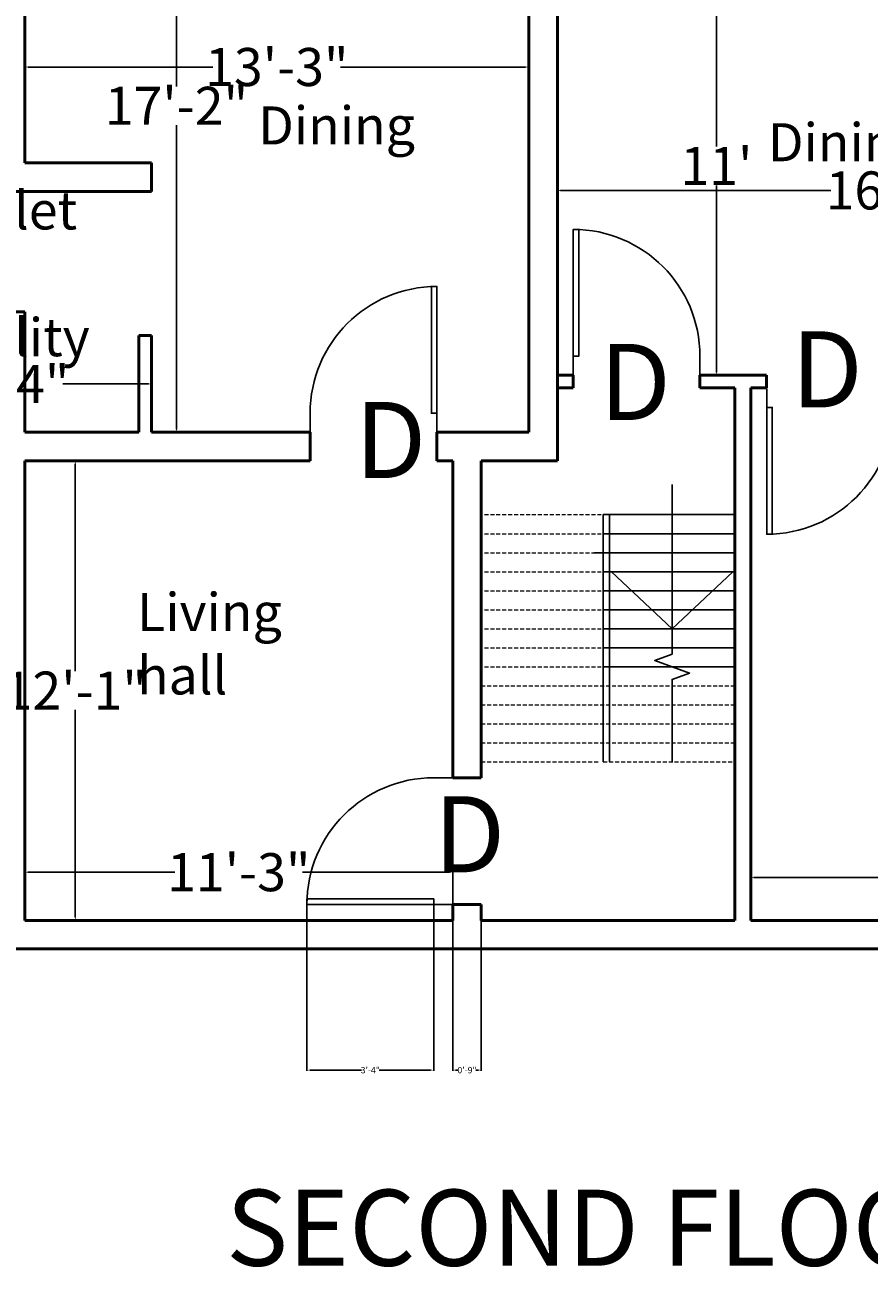
# Model space of a CAD drawing. Units: inches. Extents: x 409 to 7572, y 7 to 725.
# Tile 15 of 38: x 2984 to 3250, y 56 to 448. Entities that reach past the tile are written whole.
import ezdxf

# ---------------------------------------------------------------- set-up
doc = ezdxf.new("R2010")
doc.units = ezdxf.units.IN
doc.header["$MEASUREMENT"] = 0
doc.linetypes.add('HIDDEN', pattern=[0.375, 0.25, -0.125])
for name, color, linetype, lineweight in [('A-ANNO-DIMS', 2, 'Continuous', 18), ('A-ANNO-SYMB', 3, 'Continuous', 25), ('A-ANNO-TEXT', 7, 'Continuous', 35), ('A-AREA-IDEN', 7, 'Continuous', 25), ('A-DOOR', 3, 'Continuous', 25), ('A-FLOR-STRS', 6, 'Continuous', 25), ('A-FLOR-STRS-OVHD', 6, 'HIDDEN', 18), ('A-WALL', 7, 'Continuous', 50)]:
    doc.layers.add(name, color=color, linetype=linetype, lineweight=lineweight)
doc.styles.get("Standard").update_dxf_attribs({"font": 'arial.ttf'})
doc.dimstyles.get("Standard").update_dxf_attribs({"dimtxt": 2, "dimasz": 1, "dimexe": 0.18, "dimexo": 0.0625, "dimgap": 0.09, "dimtad": 0, "dimtih": 1, "dimtoh": 1, "dimdec": 0, "dimzin": 0, "dimdsep": 46, "dimlunit": 3, "dimtxsty": 'Standard', "dimcen": 0.09, "dimadec": 0, "dimazin": 0, "dimtfac": 1, "dimtdec": 0, "dimtofl": 0, "dimtmove": 0, "dimatfit": 3, "dimfxl": 1, "dimtolj": 1, "dimtzin": 0, "dimarcsym": 0})

# ---------------------------------------------------------------- blocks, each defined once
blk = doc.blocks.new('*U2')
for p, q in [((0, 0), (0, -6)), ((-40, 0), (-40, -6))]:
    blk.add_line(p, q)
blk.add_lwpolyline([(0, 0), (0, 40), (-1.75, 40), (-1.75, 0)], close=True)
blk.add_arc((0, 0), 40, 90, 180)
blk = doc.blocks.new('*U3')
for p, q in [((0, 0), (0, -6)), ((40, 0), (40, -6))]:
    blk.add_line(p, q)
blk.add_lwpolyline([(0, 0), (0, 40), (1.75, 40), (1.75, 0)], close=True)
blk.add_arc((0, 0), 40, 0, 90)
blk = doc.blocks.new('*U4')
for p, q in [((0, 0), (0, -6)), ((40, 0), (40, -6))]:
    blk.add_line(p, q)
blk.add_lwpolyline([(0, 0), (0, 40), (1.75, 40), (1.75, 0)], close=True)
blk.add_arc((0, 0), 40, 0, 90)
blk = doc.blocks.new('*U5')
for p, q in [((0, 0), (0, 6)), ((40, 0), (40, 6))]:
    blk.add_line(p, q)
blk.add_lwpolyline([(0, 0), (0, -40), (1.75, -40), (1.75, 0)], close=True)
blk.add_arc((0, 0), 40, 270, 0)
blk = doc.blocks.new('*D68')
at = {"layer": 'A-ANNO-DIMS', "color": 0, "lineweight": -2, "transparency": 16777216}
for p, q in [((3213.1, 165.59), (3213.1, 179.18)), ((3214.1, 179), (3260.96, 179)), ((3348.1, 179), (3301.23, 179)), ((3349.1, 165.59), (3349.1, 179.18))]:
    blk.add_line(p, q, dxfattribs=at)
at = {"layer": 'A-ANNO-DIMS', "color": 0, "transparency": 16777216}
for points in [[(3214.1, 179.16), (3214.1, 178.83), (3213.1, 179)], [(3348.1, 179.16), (3348.1, 178.83), (3349.1, 179)]]:
    blk.add_solid(points, dxfattribs=at)
at = {"layer": 'DEFPOINTS', "color": 0, "transparency": 16777216}
for p in [(3349.1, 179), (3213.1, 165.53), (3349.1, 165.53)]:
    blk.add_point(p, dxfattribs=at)
at = {"layer": 'A-ANNO-DIMS', "color": 0, "transparency": 16777216, "insert": (3281.1, 179), "char_height": 2, "attachment_point": 5}
blk.add_mtext('\\A1;{\\H6x;11\'-4"}', dxfattribs=at)
blk = doc.blocks.new('*D69')
at = {"layer": 'A-ANNO-DIMS', "color": 0, "lineweight": -2, "transparency": 16777216}
for p, q in [((2984.1, 165.59), (2984.1, 180.91)), ((2985.1, 180.73), (3031.46, 180.73)), ((3118.1, 180.73), (3071.73, 180.73)), ((3119.1, 165.59), (3119.1, 180.91))]:
    blk.add_line(p, q, dxfattribs=at)
at = {"layer": 'A-ANNO-DIMS', "color": 0, "transparency": 16777216}
for points in [[(2985.1, 180.9), (2985.1, 180.56), (2984.1, 180.73)], [(3118.1, 180.9), (3118.1, 180.56), (3119.1, 180.73)]]:
    blk.add_solid(points, dxfattribs=at)
at = {"layer": 'DEFPOINTS', "color": 0, "transparency": 16777216}
for p in [(3119.1, 180.73), (2984.1, 165.53), (3119.1, 165.53)]:
    blk.add_point(p, dxfattribs=at)
at = {"layer": 'A-ANNO-DIMS', "color": 0, "transparency": 16777216, "insert": (3051.6, 180.73), "char_height": 2, "attachment_point": 5}
blk.add_mtext('\\A1;{\\H6x;11\'-3"}', dxfattribs=at)
blk = doc.blocks.new('*D70')
at = {"layer": 'A-ANNO-DIMS', "color": 0, "lineweight": -2, "transparency": 16777216}
for p, q in [((2984.16, 310.53), (3000.2, 310.53)), ((3000.02, 309.53), (3000.02, 244.15)), ((3000.02, 166.53), (3000.02, 231.92)), ((2984.16, 165.53), (3000.2, 165.53))]:
    blk.add_line(p, q, dxfattribs=at)
at = {"layer": 'A-ANNO-DIMS', "color": 0, "transparency": 16777216}
for points in [[(2999.85, 309.53), (3000.19, 309.53), (3000.02, 310.53)], [(2999.85, 166.53), (3000.19, 166.53), (3000.02, 165.53)]]:
    blk.add_solid(points, dxfattribs=at)
at = {"layer": 'DEFPOINTS', "color": 0, "transparency": 16777216}
for p in [(2984.1, 310.53), (2984.1, 165.53), (3000.02, 165.53)]:
    blk.add_point(p, dxfattribs=at)
at = {"layer": 'A-ANNO-DIMS', "color": 0, "transparency": 16777216, "insert": (3000.02, 238.03), "char_height": 2, "attachment_point": 5}
blk.add_mtext('\\A1;{\\H6x;12\'-1"}', dxfattribs=at)
blk = doc.blocks.new('*D82')
at = {"layer": 'A-ANNO-DIMS', "color": 0, "lineweight": -2, "transparency": 16777216}
for p, q in [((2984.1, 404.59), (2984.1, 434.95)), ((2985.1, 434.77), (3043.46, 434.77)), ((3142.1, 434.77), (3083.73, 434.77)), ((3143.1, 404.59), (3143.1, 434.95))]:
    blk.add_line(p, q, dxfattribs=at)
at = {"layer": 'A-ANNO-DIMS', "color": 0, "transparency": 16777216}
for points in [[(2985.1, 434.93), (2985.1, 434.6), (2984.1, 434.77)], [(3142.1, 434.93), (3142.1, 434.6), (3143.1, 434.77)]]:
    blk.add_solid(points, dxfattribs=at)
at = {"layer": 'DEFPOINTS', "color": 0, "transparency": 16777216}
for p in [(3143.1, 434.77), (2984.1, 404.53), (3143.1, 404.53)]:
    blk.add_point(p, dxfattribs=at)
at = {"layer": 'A-ANNO-DIMS', "color": 0, "transparency": 16777216, "insert": (3063.6, 434.77), "char_height": 2, "attachment_point": 5}
blk.add_mtext('\\A1;{\\H6x;13\'-3"}', dxfattribs=at)
blk = doc.blocks.new('*D83')
at = {"layer": 'A-ANNO-DIMS', "color": 0, "lineweight": -2, "transparency": 16777216}
for p, q in [((3041.04, 525.53), (3031.75, 525.53)), ((3031.93, 524.53), (3031.93, 428.65)), ((3031.93, 320.53), (3031.93, 416.42)), ((3049.04, 319.53), (3031.75, 319.53))]:
    blk.add_line(p, q, dxfattribs=at)
at = {"layer": 'A-ANNO-DIMS', "color": 0, "transparency": 16777216}
for points in [[(3031.77, 524.53), (3032.1, 524.53), (3031.93, 525.53)], [(3031.77, 320.53), (3032.1, 320.53), (3031.93, 319.53)]]:
    blk.add_solid(points, dxfattribs=at)
at = {"layer": 'DEFPOINTS', "color": 0, "transparency": 16777216}
for p in [(3041.1, 525.53), (3031.93, 319.53), (3049.1, 319.53)]:
    blk.add_point(p, dxfattribs=at)
at = {"layer": 'A-ANNO-DIMS', "color": 0, "transparency": 16777216, "insert": (3031.93, 422.53), "char_height": 2, "attachment_point": 5}
blk.add_mtext('\\A1;{\\H6x;17\'-2"}', dxfattribs=at)
blk = doc.blocks.new('*D80')
at = {"layer": 'A-ANNO-DIMS', "color": 0, "lineweight": -2, "transparency": 16777216}
for p, q in [((3152.1, 403.47), (3152.1, 395.65)), ((3344.1, 403.47), (3344.1, 395.65)), ((3153.1, 395.83), (3238.39, 395.83)), ((3343.1, 395.83), (3257.81, 395.83))]:
    blk.add_line(p, q, dxfattribs=at)
at = {"layer": 'A-ANNO-DIMS', "color": 0, "transparency": 16777216}
for points in [[(3153.1, 396), (3153.1, 395.66), (3152.1, 395.83)], [(3343.1, 396), (3343.1, 395.66), (3344.1, 395.83)]]:
    blk.add_solid(points, dxfattribs=at)
at = {"layer": 'DEFPOINTS', "color": 0, "transparency": 16777216}
for p in [(3152.1, 403.53), (3344.1, 403.53), (3344.1, 395.83)]:
    blk.add_point(p, dxfattribs=at)
at = {"layer": 'A-ANNO-DIMS', "color": 0, "transparency": 16777216, "insert": (3248.1, 395.83), "char_height": 2, "attachment_point": 5}
blk.add_mtext("\\A1;{\\H6x;16'}", dxfattribs=at)
blk = doc.blocks.new('*D84')
at = {"layer": 'A-ANNO-DIMS', "color": 0, "lineweight": -2, "transparency": 16777216}
for p, q in [((3206.36, 469.53), (3202.12, 469.53)), ((3202.3, 468.53), (3202.3, 409.65)), ((3202.3, 338.53), (3202.3, 397.42)), ((3207.54, 337.53), (3202.12, 337.53))]:
    blk.add_line(p, q, dxfattribs=at)
at = {"layer": 'A-ANNO-DIMS', "color": 0, "transparency": 16777216}
for points in [[(3202.13, 468.53), (3202.46, 468.53), (3202.3, 469.53)], [(3202.13, 338.53), (3202.46, 338.53), (3202.3, 337.53)]]:
    blk.add_solid(points, dxfattribs=at)
at = {"layer": 'DEFPOINTS', "color": 0, "transparency": 16777216}
for p in [(3206.42, 469.53), (3202.3, 337.53), (3207.6, 337.53)]:
    blk.add_point(p, dxfattribs=at)
at = {"layer": 'A-ANNO-DIMS', "color": 0, "transparency": 16777216, "insert": (3202.3, 403.53), "char_height": 2, "attachment_point": 5}
blk.add_mtext("\\A1;{\\H6x;11'}", dxfattribs=at)
blk = doc.blocks.new('*D89')
at = {"layer": 'A-ANNO-DIMS', "color": 0, "lineweight": -2, "transparency": 16777216}
for p, q in [((2936.1, 346.33), (2936.1, 334.6)), ((3024.1, 346.33), (3024.1, 334.6)), ((2937.1, 334.78), (2964.11, 334.78)), ((3023.1, 334.78), (2996.09, 334.78))]:
    blk.add_line(p, q, dxfattribs=at)
at = {"layer": 'A-ANNO-DIMS', "color": 0, "transparency": 16777216}
for points in [[(2937.1, 334.95), (2937.1, 334.61), (2936.1, 334.78)], [(3023.1, 334.95), (3023.1, 334.61), (3024.1, 334.78)]]:
    blk.add_solid(points, dxfattribs=at)
at = {"layer": 'DEFPOINTS', "color": 0, "transparency": 16777216}
for p in [(2936.1, 346.39), (3024.1, 346.39), (3024.1, 334.78)]:
    blk.add_point(p, dxfattribs=at)
at = {"layer": 'A-ANNO-DIMS', "color": 0, "transparency": 16777216, "insert": (2980.1, 334.78), "char_height": 2, "attachment_point": 5}
blk.add_mtext('\\A1;{\\H6x;7\'-4"}', dxfattribs=at)
blk = doc.blocks.new('*D184')
at = {"layer": 'A-ANNO-DIMS', "color": 0, "lineweight": -2, "transparency": 16777216}
for p, q in [((3119.1, 165.47), (3119.1, 118.1)), ((3128.1, 165.47), (3128.1, 118.1)), ((3120.1, 118.28), (3120.85, 118.28)), ((3127.1, 118.28), (3126.35, 118.28))]:
    blk.add_line(p, q, dxfattribs=at)
at = {"layer": 'A-ANNO-DIMS', "color": 0, "transparency": 16777216}
for points in [[(3120.1, 118.45), (3120.1, 118.11), (3119.1, 118.28)], [(3127.1, 118.45), (3127.1, 118.11), (3128.1, 118.28)]]:
    blk.add_solid(points, dxfattribs=at)
at = {"layer": 'DEFPOINTS', "color": 0, "transparency": 16777216}
for p in [(3119.1, 165.53), (3128.1, 165.53), (3128.1, 118.28)]:
    blk.add_point(p, dxfattribs=at)
at = {"layer": 'A-ANNO-DIMS', "color": 0, "transparency": 16777216, "insert": (3123.6, 118.28), "char_height": 2, "attachment_point": 5}
blk.add_mtext('\\A1;0\'-9"', dxfattribs=at)
blk = doc.blocks.new('*D187')
at = {"layer": 'A-ANNO-DIMS', "color": 0, "lineweight": -2, "transparency": 16777216}
for p, q in [((3073.1, 170.47), (3073.1, 118.1)), ((3113.1, 170.47), (3113.1, 118.1)), ((3074.1, 118.28), (3090.35, 118.28)), ((3112.1, 118.28), (3095.85, 118.28))]:
    blk.add_line(p, q, dxfattribs=at)
at = {"layer": 'A-ANNO-DIMS', "color": 0, "transparency": 16777216}
for points in [[(3074.1, 118.45), (3074.1, 118.11), (3073.1, 118.28)], [(3112.1, 118.45), (3112.1, 118.11), (3113.1, 118.28)]]:
    blk.add_solid(points, dxfattribs=at)
at = {"layer": 'DEFPOINTS', "color": 0, "transparency": 16777216}
for p in [(3073.1, 170.53), (3113.1, 170.53), (3113.1, 118.28)]:
    blk.add_point(p, dxfattribs=at)
at = {"layer": 'A-ANNO-DIMS', "color": 0, "transparency": 16777216, "insert": (3093.1, 118.28), "char_height": 2, "attachment_point": 5}
blk.add_mtext('\\A1;3\'-4"', dxfattribs=at)

msp = doc.modelspace()

# ---------------------------------------------------------------- linework, layer by layer
at = {"layer": 'A-FLOR-STRS'}
for p, q in [((3188.3, 303.06), (3188.3, 257.53)), ((3166.6, 293.53), (3208.1, 293.53)), ((3166.6, 293.53), (3166.6, 215.53)), ((3168.6, 293.53), (3168.6, 215.53)), ((3166.6, 287.53), (3208.1, 287.53)), ((3163.76, 281.53), (3208.1, 281.53)), ((3166.6, 275.53), (3208.1, 275.53)), ((3188.3, 257.53), (3169.18, 275.53)), ((3188.3, 257.53), (3207.43, 275.53)), ((3166.6, 269.53), (3208.1, 269.53)), ((3166.6, 263.53), (3208.1, 263.53)), ((3166.6, 257.53), (3208.1, 257.53)), ((3166.6, 251.53), (3208.1, 251.53)), ((3166.6, 245.53), (3208.1, 245.53))]:
    msp.add_line(p, q, dxfattribs=at)
msp.add_lwpolyline([(3188.3, 257.71), (3188.3, 249.53), (3182.81, 247.53), (3193.8, 243.53), (3188.3, 241.53), (3188.3, 215.35)], dxfattribs=at)
at = {"layer": 'A-FLOR-STRS-OVHD', "ltscale": 5}
for p, q in [((3129.1, 293.53), (3166.6, 293.53)), ((3129.1, 287.53), (3166.6, 287.53)), ((3129.1, 281.53), (3163.76, 281.53)), ((3129.1, 275.53), (3166.6, 275.53)), ((3129.1, 269.53), (3166.6, 269.53)), ((3129.1, 263.53), (3166.6, 263.53)), ((3129.1, 257.53), (3166.6, 257.53)), ((3129.1, 251.53), (3166.6, 251.53)), ((3129.1, 245.53), (3166.6, 245.53)), ((3128.1, 239.53), (3208.1, 239.53)), ((3128.1, 233.53), (3208.1, 233.53)), ((3128.1, 227.53), (3208.1, 227.53)), ((3128.1, 221.53), (3208.1, 221.53)), ((3128.1, 215.53), (3165.6, 215.53)), ((3166.6, 215.53), (3208.1, 215.53))]:
    msp.add_line(p, q, dxfattribs=at)
at = {"layer": 'A-WALL'}
for p, q in [((2984.1, 525.53), (2984.1, 404.53)), ((3143.1, 525.53), (3143.1, 319.53)), ((3152.1, 469.53), (3152.1, 337.53)), ((3024.1, 404.53), (2984.1, 404.53)), ((3024.1, 404.53), (3024.1, 395.53)), ((2984.1, 395.53), (2936.1, 395.53)), ((3024.1, 395.53), (2984.1, 395.53)), ((2984.1, 357.53), (2975.1, 357.53)), ((2984.1, 357.53), (2984.1, 319.53)), ((3020.1, 350.03), (3020.1, 319.53)), ((3024.1, 350.03), (3020.1, 350.03)), ((3024.1, 350.03), (3024.1, 319.53)), ((3152.1, 337.53), (3157.1, 337.53)), ((3152.1, 337.53), (3152.1, 333.53)), ((3157.1, 337.53), (3157.1, 333.53)), ((3197.1, 337.53), (3218.1, 337.53)), ((3197.1, 337.53), (3197.1, 333.53)), ((3218.1, 333.53), (3218.1, 337.53)), ((3152.1, 333.53), (3157.1, 333.53)), ((3152.1, 333.53), (3152.1, 310.53)), ((3197.1, 333.53), (3208.1, 333.53)), ((3208.1, 333.53), (3208.1, 165.53)), ((3213.1, 333.53), (3218.1, 333.53)), ((3213.1, 333.53), (3213.1, 165.53)), ((3020.1, 319.53), (2984.1, 319.53)), ((3074.1, 319.53), (3024.1, 319.53)), ((3074.1, 319.53), (3074.1, 310.53)), ((3143.1, 319.53), (3114.1, 319.53)), ((3114.1, 310.53), (3114.1, 319.53)), ((3074.1, 310.53), (2984.1, 310.53)), ((2984.1, 310.53), (2984.1, 165.53)), ((3119.1, 310.53), (3114.1, 310.53)), ((3119.1, 310.53), (3119.1, 210.53)), ((3152.1, 310.53), (3128.1, 310.53)), ((3128.1, 310.53), (3128.1, 210.53)), ((3119.1, 210.53), (3128.1, 210.53)), ((3119.1, 170.53), (3119.1, 165.53)), ((3128.1, 170.53), (3119.1, 170.53)), ((3128.1, 170.53), (3128.1, 165.53)), ((2984.1, 165.53), (3119.1, 165.53)), ((3128.1, 165.53), (3208.1, 165.53)), ((3213.1, 165.53), (3349.1, 165.53)), ((2975.1, 156.53), (3349.1, 156.53))]:
    msp.add_line(p, q, dxfattribs=at)

# ---------------------------------------------------------------- block references
at = {"layer": 'A-DOOR'}
for name, p in [('*U4', (3157.1, 343.53)), ('*U2', (3114.1, 325.53)), ('*U5', (3218.16, 327.37))]:
    msp.add_blockref(name, p, dxfattribs=at)
at = {"layer": 'A-DOOR', "rotation": 90}
msp.add_blockref('*U3', (3113.1, 170.53), dxfattribs=at)

# ---------------------------------------------------------------- texts
at = {"layer": 'A-ANNO-SYMB', "char_height": 24, "attachment_point": 1}
for insert in [(3225.93, 351.37), (3165.39, 347.4), (3088.23, 329.09), (3113.1, 204.69)]:
    msp.add_mtext_dynamic_manual_height_columns('D', width=19.1972, gutter_width=1, heights=[0], dxfattribs=dict(at, insert=insert))
at = {"layer": 'A-ANNO-TEXT', "insert": (3047.61, 80.54), "char_height": 24, "attachment_point": 1}
msp.add_mtext_dynamic_manual_height_columns('SECOND FLOOR', width=577.2242, gutter_width=1, heights=[0], dxfattribs=at)
at = {"layer": 'A-AREA-IDEN', "char_height": 12, "attachment_point": 1}
for s, width, insert in [('Dining ', 67.5069, (3057.71, 422.33)), ('Dining ', 67.5069, (3218.53, 417.03)), ('toilet / utility', 49.2946, (2960.1, 395.53)), ('Living hall', 58.8843, (3019.52, 268.81))]:
    msp.add_mtext_dynamic_manual_height_columns(s, width=width, gutter_width=1, heights=[0], dxfattribs=dict(at, insert=insert))

# ---------------------------------------------------------------- dimensions: what is measured, and where the dimension line sits
at = {"layer": 'A-ANNO-DIMS'}
dim = msp.add_linear_dim(base=(3031.93, 319.53), p1=(3041.1, 525.53), p2=(3049.1, 319.53), angle=90, text='{\\H6x;<>}', dimstyle='Standard', override={"dimclrd": 0, "dimclre": 0, "dimclrt": 0}, dxfattribs=at)
dim.commit()
dim.dimension.update_dxf_attribs({"geometry": '*D83', "text_midpoint": (3031.93, 422.53), "dimtype": 160})
for base, p1, p2, picture, middle in [((3202.3, 337.53), (3206.42, 469.53), (3207.6, 337.53), '*D84', (3202.3, 403.53)), ((3000.02, 165.53), (2984.1, 310.53), (2984.1, 165.53), '*D70', (3000.02, 238.03))]:
    dim = msp.add_linear_dim(base=base, p1=p1, p2=p2, angle=90, text='{\\H6x;<>}', dimstyle='Standard', override={"dimclrd": 0, "dimclre": 0, "dimclrt": 0}, dxfattribs=at)
    dim.commit()
    dim.dimension.update_dxf_attribs({"geometry": picture, "text_midpoint": middle})
for base, p1, p2, picture, middle in [((3143.1, 434.77), (2984.1, 404.53), (3143.1, 404.53), '*D82', (3063.6, 434.77)), ((3024.1, 334.78), (2936.1, 346.39), (3024.1, 346.39), '*D89', (2980.1, 334.78)), ((3119.1, 180.73), (2984.1, 165.53), (3119.1, 165.53), '*D69', (3051.6, 180.73)), ((3349.1, 179), (3213.1, 165.53), (3349.1, 165.53), '*D68', (3281.1, 179))]:
    dim = msp.add_linear_dim(base=base, p1=p1, p2=p2, text='{\\H6x;<>}', dimstyle='Standard', override={"dimclrd": 0, "dimclre": 0, "dimclrt": 0}, dxfattribs=at)
    dim.commit()
    dim.dimension.update_dxf_attribs({"geometry": picture, "text_midpoint": middle})
dim = msp.add_linear_dim(base=(3344.1, 395.83), p1=(3152.1, 403.53), p2=(3344.1, 403.53), text='{\\H6x;<>}', dimstyle='Standard', override={"dimclrd": 0, "dimclre": 0, "dimclrt": 0}, dxfattribs=at)
dim.commit()
dim.dimension.update_dxf_attribs({"geometry": '*D80', "text_midpoint": (3248.1, 395.83), "dimtype": 160})
for base, p1, p2, picture, middle in [((3113.1, 118.28), (3073.1, 170.53), (3113.1, 170.53), '*D187', (3093.1, 118.28)), ((3128.1, 118.28), (3119.1, 165.53), (3128.1, 165.53), '*D184', (3123.6, 118.28))]:
    dim = msp.add_linear_dim(base=base, p1=p1, p2=p2, dimstyle='Standard', override={"dimdec": 1, "dimlfac": 1, "dimrnd": 0, "dimzin": 1, "dimdsep": 46, "dimlunit": 4, "dimfrac": 2}, dxfattribs=at)
    dim.commit()
    dim.dimension.update_dxf_attribs({"geometry": picture, "text_midpoint": middle})

doc.saveas('drawing.dxf')
